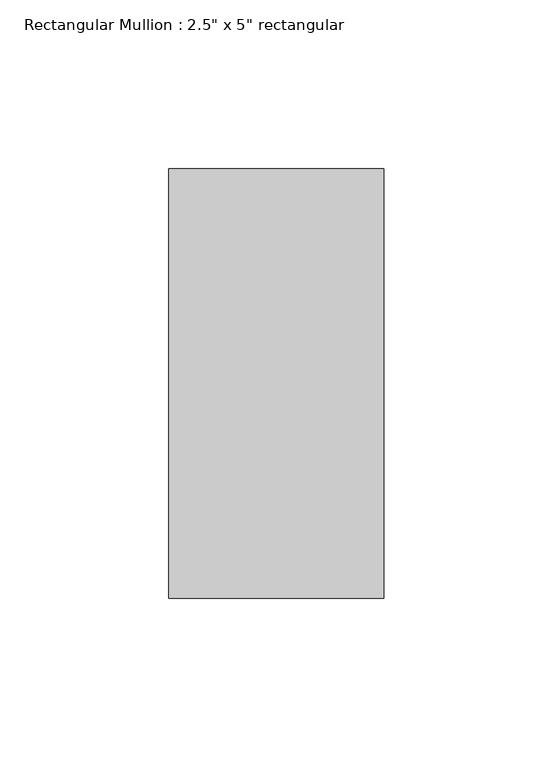
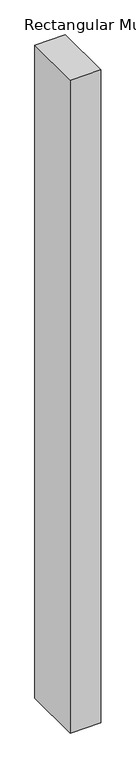
"""IFC4 building model written with IfcOpenShell, lengths in millimetres: member geometry."""

from ifc_helpers import new_model, si_unit, frame, origin, place, context, project, spatial, polyline, outline, extrude, source, transform, mapped, element, save


def member_b1e1b578(model_context):
    return source(origin(), model_context, "Body", "SweptSolid", [
        extrude(outline(polyline([(31.75, 63.5), (31.75, -63.5), (-31.75, -63.5), (-31.75, 63.5), (31.75, 63.5)])), frame((0.0, 0.0, -1433.7701004), z_axis=(0.0, 0.0, 1.0), x_axis=(1.0, 0.0, 0.0)), (0.0, 0.0, 1.0), 1433.7701004),
    ])


if __name__ == "__main__":
    model = new_model("IFC4")
    model_context = context("Model", 3, world=origin())
    ifc_project = project(units=[si_unit("LENGTHUNIT", "METRE", prefix="MILLI")], contexts=[model_context])
    site = spatial("IfcSite", under=ifc_project)
    building = spatial("IfcBuilding", under=site)
    placement = place(None, origin())
    member_shape = member_b1e1b578(model_context)
    element("IfcMember", 1, ObjectType="Rectangular Mullion : 2.5\" x 5\" rectangular", at=placement, inside=building, context=model_context, shape_type="MappedRepresentation", body=[
        mapped(member_shape, transform((0.0, 0.0, 0.0), x_axis=(1.0, 0.0, 0.0), y_axis=(0.0, 1.0, 0.0), z_axis=(0.0, 0.0, 1.0))),
    ])
    save(model, "model.ifc")

# Revit data of these elements
# Type "Rectangular Mullion : 2.5\" x 5\" rectangular"
#   built-in parameter 1007304 = 0.416667 (stored number, unit not read)
#   built-in parameter 1007301 = 0.104167 (stored number, unit not read)
#   built-in parameter 1007300 = 0.104167 (stored number, unit not read)
# Element 1 (IfcMember, "Rectangular Mullion : 2.5\" x 5\" rectangular")
#   Materials on its faces: "Aluminum"
# Materials
#   "Aluminum": class "Metal", colour RGB 247 247 247, transparency 0, Description = "Aluminum 6061", Cost = 0
